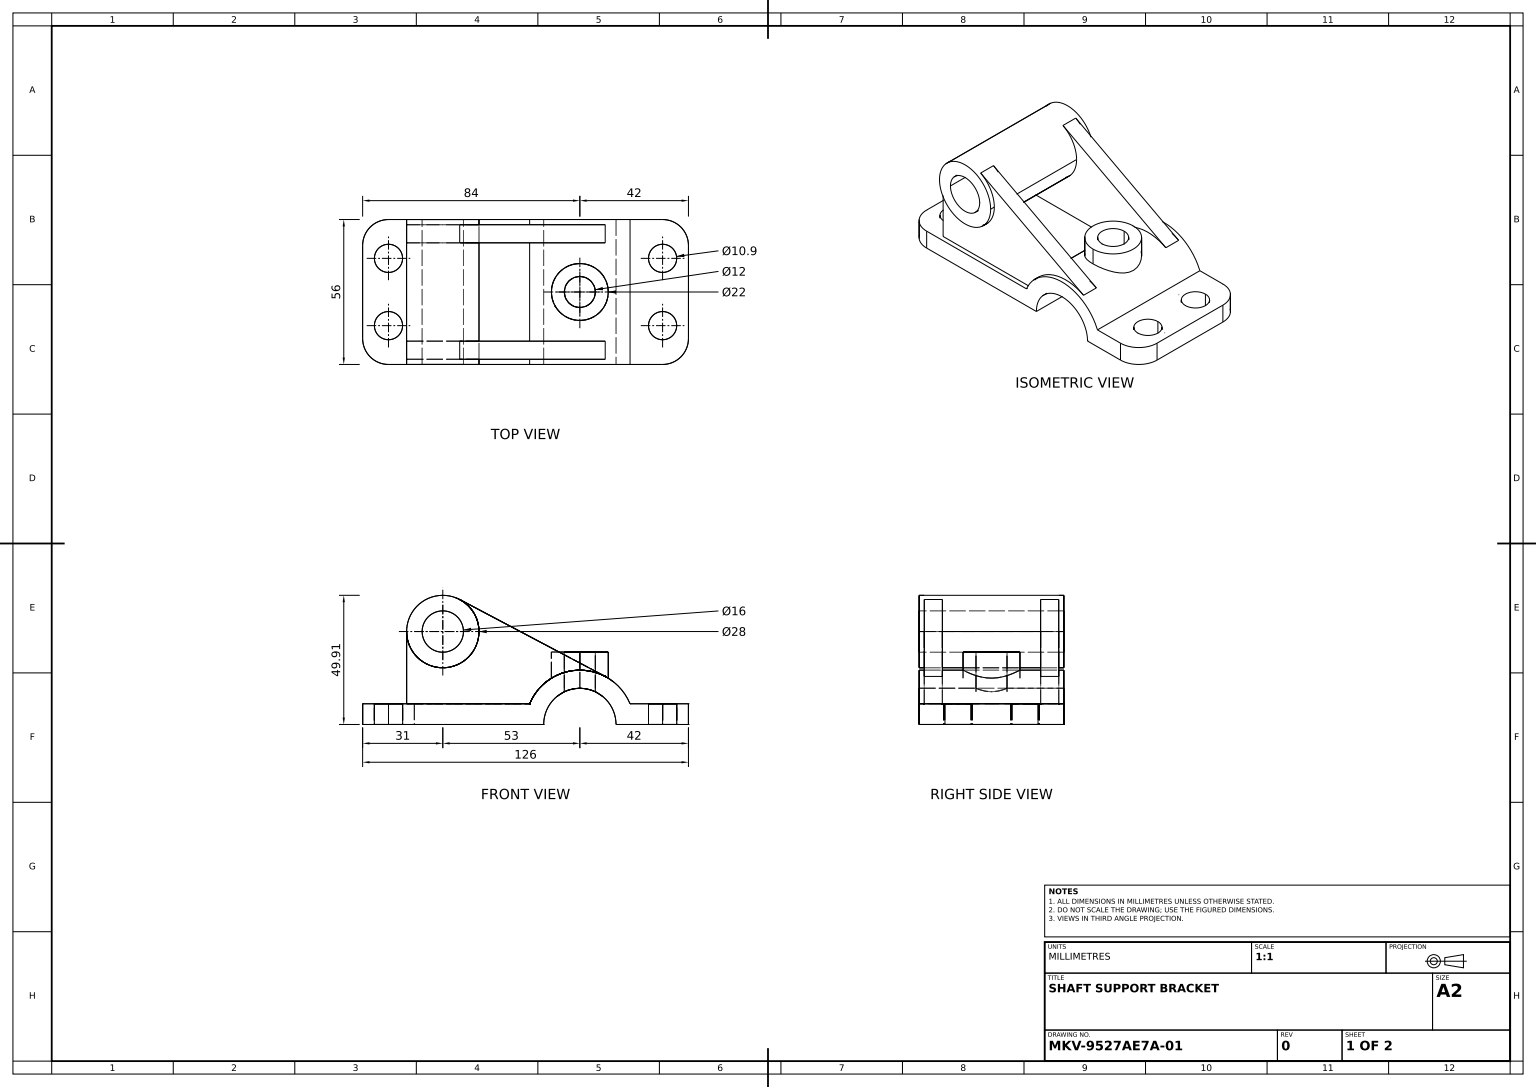
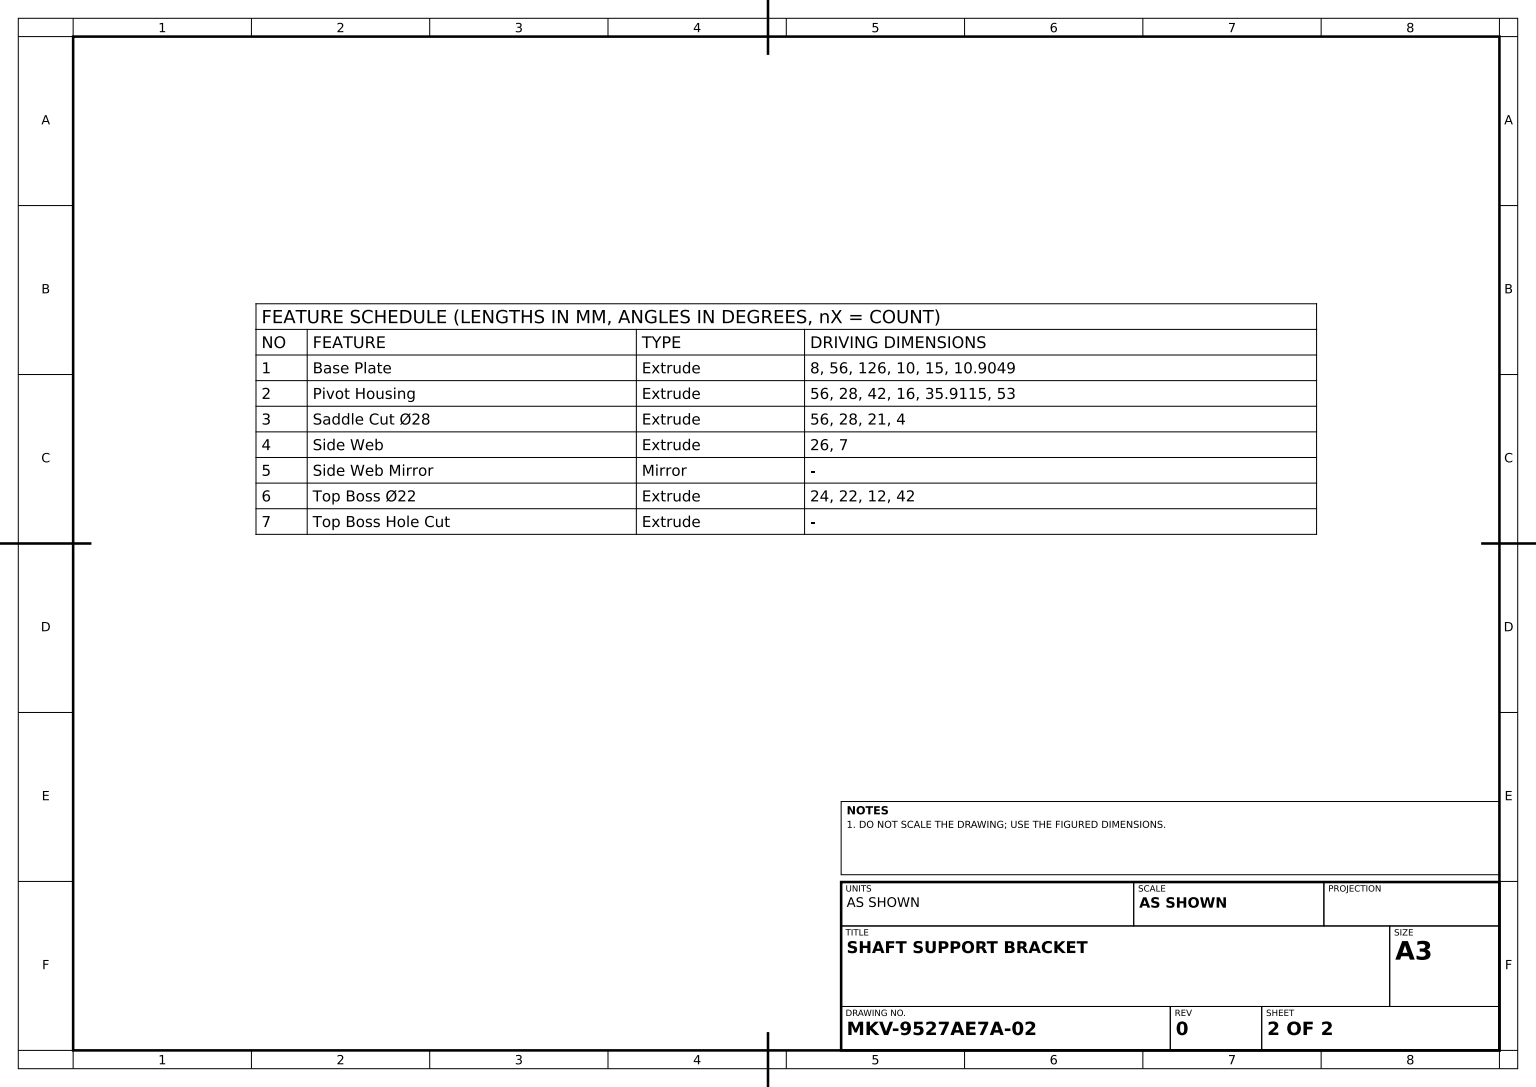
from build123d import *
from build123d.topology import SkipClean

# Parameters (mm, degrees)
BASE_PLATE_SKETCH_R      = 5.452465884
BASE_PLATE_DEPTH         = 4
PIVOT_HOUSING_SKETCH_R   = 14
PIVOT_HOUSING_SKETCH_R_2 = 8
PIVOT_HOUSING_DEPTH      = 28
SADDLE_CUT_SKETCH_R      = 14
SADDLE_CUT_28_DEPTH      = 28
SIDE_WEB_SKETCH_R        = 8
SIDE_WEB_DEPTH           = 7
TOP_BOSS_22_REACH        = 76.411
TOP_BOSS_22_END_RADIUS   = 21
TOP_BOSS_SKETCH_R        = 11
TOP_BOSS_SKETCH_R_2      = 6
TOP_BOSS_HOLE_CUT_REACH  = 76.411
TOP_BOSS_HOLE_SKETCH_R   = 6


with BuildPart() as part:
    # Base Plate Sketch → Base Plate (new, symmetric)
    with BuildSketch(Plane(origin=(0, 0, 0), x_dir=(1, 0, 0), z_dir=(0, 1, 0))):
        with BuildLine():
            Line((-53, 28), (53, 28))
            ThreePointArc((53, 28), (60.071067812, 25.071067812), (63, 18))
            Line((63, 18), (63, -18))
            ThreePointArc((63, -18), (60.071067812, -25.071067812), (53, -28))
            Line((53, -28), (-53, -28))
            ThreePointArc((-53, -28), (-60.071067812, -25.071067812), (-63, -18))
            Line((-63, -18), (-63, 18))
            ThreePointArc((-63, 18), (-60.071067812, 25.071067812), (-53, 28))
        make_face()
        with Locations(Location((-53, 13, 0), (0, 0, 270))):
            Circle(BASE_PLATE_SKETCH_R, mode=Mode.SUBTRACT)
        with Locations(Location((-53, -13, 0), (0, 0, 90))):
            Circle(BASE_PLATE_SKETCH_R, mode=Mode.SUBTRACT)
        with Locations(Location((53, -13, 0), (0, 0, 270))):
            Circle(BASE_PLATE_SKETCH_R, mode=Mode.SUBTRACT)
        with Locations(Location((53, 13, 0), (0, 0, 90))):
            Circle(BASE_PLATE_SKETCH_R, mode=Mode.SUBTRACT)
    extrude(amount=BASE_PLATE_DEPTH, both=True)

    # Pivot Housing Sketch → Pivot Housing (add, symmetric)
    # profile 1 of 2: a face of its own
    with BuildSketch(Plane.XY):
        with Locations((-32, 31.911479001)):
            Circle(PIVOT_HOUSING_SKETCH_R)
        with Locations((-32, 31.911479001)):
            Circle(PIVOT_HOUSING_SKETCH_R_2, mode=Mode.SUBTRACT)
    # profile 2 of 2: a face of its own
    with BuildSketch(Plane.XY):
        with BuildLine():
            Line((0, -4), (7, -4))
            ThreePointArc((7, -4), (21, 10), (35, -4))
            Line((35, -4), (42, -4))
            ThreePointArc((42, -4), (21, 17), (0, -4))
        make_face()
    extrude(amount=PIVOT_HOUSING_DEPTH, both=True)


with BuildPart() as pivot_housing_piece_1:
    # of the separate pieces the step leaves, piece 1, a body of its own (pivot_housing_pieces)
    add(part.part.solids().sort_by_distance((-53, -4, -28))[0])

    # Saddle Cut Sketch → Saddle Cut Ø28 (cut, symmetric)
    with SkipClean():  # the faces are left unmerged after this step: merging them gives an invalid solid
        with BuildSketch(Plane.XY):
            with Locations((21, -4)):
                Circle(SADDLE_CUT_SKETCH_R)
        extrude(amount=SADDLE_CUT_28_DEPTH, both=True, mode=Mode.SUBTRACT)



with BuildPart() as pivot_housing_piece_2:
    # of the separate pieces the step leaves, piece 2, a body of its own (pivot_housing_pieces)
    add(part.part.solids().sort_by_distance((-18, 31.911479001, -28))[0])


with BuildPart() as pivot_housing_piece_1_1:
    with SkipClean():  # the faces are left unmerged after this step: merging them gives an invalid solid
        add(pivot_housing_piece_1.part)

        add(pivot_housing_piece_2.part)  # Side Web merges Pivot Housing piece 2
        # Side Web Sketch → Side Web (add)
        with BuildSketch(Plane.XY.offset(26)):
            with BuildLine():
                Line((-46, 4), (1.583512161, 4))
                ThreePointArc((1.583512161, 4), (13.858235624, 15.748296169), (30.808163701, 14.568788997))
                Line((30.808163701, 14.568788997), (-25.4612242, 44.290671665))
                ThreePointArc((-25.4612242, 44.290671665), (-39.22693361, 43.901951494), (-46, 31.911479001))
                Line((-46, 31.911479001), (-46, 4))
            make_face()
            with Locations((-32, 31.911479001)):
                Circle(SIDE_WEB_SKETCH_R, mode=Mode.SUBTRACT)
        side_web = extrude(amount=-SIDE_WEB_DEPTH)

    # Side Web Mirror: Side Web across plane
    with SkipClean():  # the faces are left unmerged after this step: merging them gives an invalid solid
        add(side_web.mirror(Plane.XY))

    # Top Boss Ø22: up to this cylinder (the profile starts outside it)
    with SkipClean():  # the faces are left unmerged after this step: merging them gives an invalid solid
        top_boss_22_end = Plane(origin=(21, -4, -10.688873), z_dir=(0, 0, -1)) * Cylinder(TOP_BOSS_22_END_RADIUS, 195.822, mode=Mode.PRIVATE)
        # Top Boss Sketch → Top Boss Ø22 (add, up to the surface)
        with BuildSketch(Plane(origin=(0, 24, 0), x_dir=(1, 0, 0), z_dir=(0, 1, 0)), mode=Mode.PRIVATE) as top_boss_22_sk1:
            with Locations(Location((21, 0, 0), (0, 0, 270))):
                Circle(TOP_BOSS_SKETCH_R)
            with Locations(Location((21, 0, 0), (0, 0, 270))):
                Circle(TOP_BOSS_SKETCH_R_2, mode=Mode.SUBTRACT)
        top_boss_22_tool1 = extrude(top_boss_22_sk1.sketch, amount=-TOP_BOSS_22_REACH, mode=Mode.PRIVATE) - top_boss_22_end
        add(top_boss_22_tool1.solids().sort_by_distance((21, 24, -10.688873))[0])

    # Top Boss Hole Sketch → Top Boss Hole Cut (cut, up to next)
    with BuildSketch(Plane(origin=(0, 24, 0), x_dir=(1, 0, 0), z_dir=(0, 1, 0)), mode=Mode.PRIVATE) as top_boss_hole_cut_sk1:
        with Locations(Location((21, 0, 0), (0, 0, 270))):
            Circle(TOP_BOSS_HOLE_SKETCH_R)
    top_boss_hole_cut_tool1 = extrude(top_boss_hole_cut_sk1.sketch, amount=-TOP_BOSS_HOLE_CUT_REACH, mode=Mode.PRIVATE) & pivot_housing_piece_1_1.part
    add(top_boss_hole_cut_tool1.solids().sort_by_distance((21, 24, 0))[0], mode=Mode.SUBTRACT)


solid = pivot_housing_piece_1_1.part
